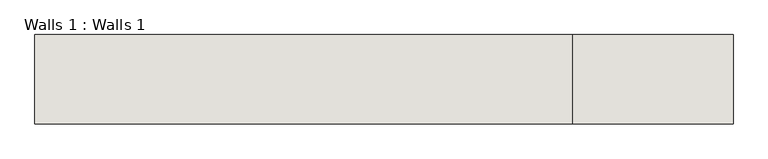
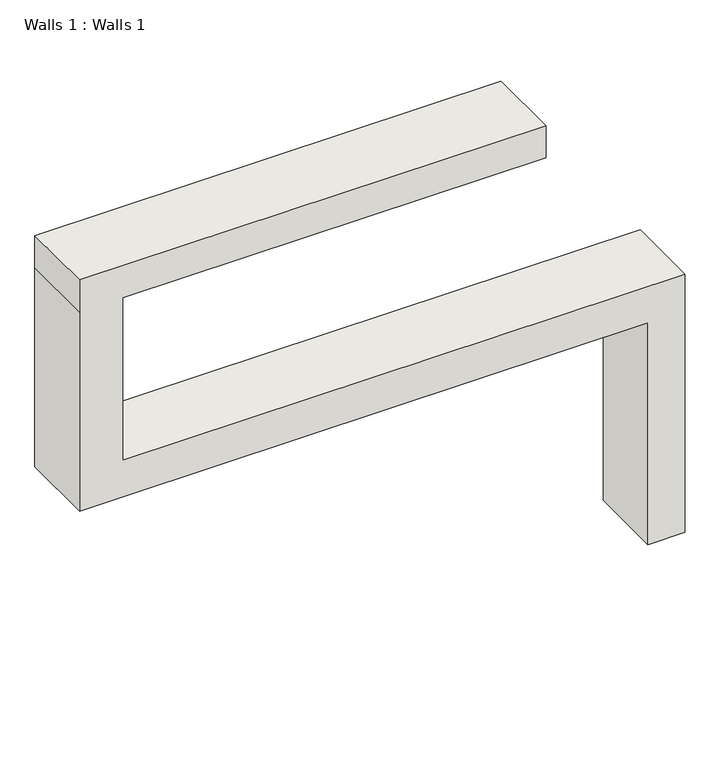
"""IFC4 building model written with IfcOpenShell, lengths in millimetres: wall geometry, Walls 1 : Walls 1."""

from ifc_helpers import new_model, si_unit, frame, origin, place, context, project, spatial, polyline, outline, extrude, source, transform, mapped, element, save


def walls_1_walls_1_5b47a2ba(model_context):
    return source(origin(), model_context, "Body", "SweptSolid", [
        extrude(outline(polyline([(7315.2, -12101.9931367), (7315.2, -5146.9687556), (7874.0, -5146.9687556), (7874.0, -12813.1931367), (7315.2, -12813.1931367), (3857.1175789, -12813.1931367), (3857.1175789, -12051.1931367), (3857.1175789, -3465.9931367), (0.0, -3465.9931367), (0.0, -2856.3931367), (3352.8, -2856.3931367), (4490.4353614, -2856.3931367), (4490.4353614, -12101.9931367), (7315.2, -12101.9931367)])), frame((0.0, 1282.1739897, 0.0), z_axis=(0.0, 1.0, 0.0), x_axis=(0.0, 0.0, 1.0)), (0.0, 0.0, 1.0), 1274.1057169),
    ])


if __name__ == "__main__":
    model = new_model("IFC4")
    model_context = context("Model", 3, world=origin())
    ifc_project = project(units=[si_unit("LENGTHUNIT", "METRE", prefix="MILLI")], contexts=[model_context])
    site = spatial("IfcSite", under=ifc_project)
    building = spatial("IfcBuilding", under=site)
    placement = place(None, origin())
    walls_1_walls_1_shape = walls_1_walls_1_5b47a2ba(model_context)
    element("IfcWall", 1, ObjectType="Walls 1 : Walls 1", at=placement, inside=building, context=model_context, shape_type="MappedRepresentation", body=[
        mapped(walls_1_walls_1_shape, transform((0.0, 0.0, 0.0), x_axis=(1.0, 0.0, 0.0), y_axis=(0.0, 1.0, 0.0), z_axis=(0.0, 0.0, 1.0))),
    ])
    save(model, "model.ifc")

# Revit data of these elements
# Element 1 (IfcWall, "Walls 1 : Walls 1")
#   Materials on its faces: "Default Wall"
# Materials
#   "Default Wall": colour RGB 128 128 128, transparency 0
